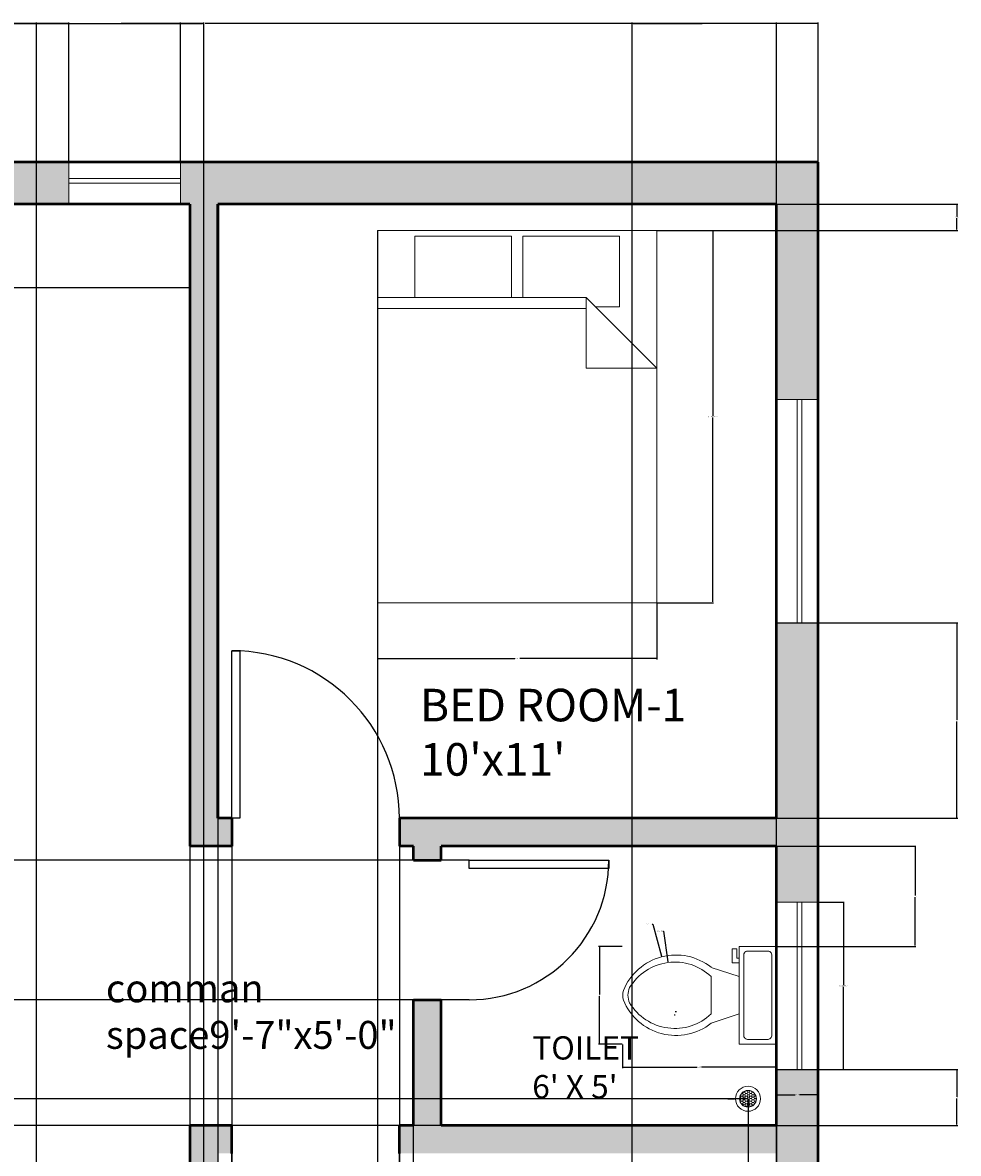
# Model space of a CAD drawing. Units: inches. Extents: x 1489 to 1813, y 1703 to 2293.
# Tile 4 of 4: x 1612 to 1813, y 2050 to 2293. Entities that reach past the tile are written whole.
import ezdxf

# ---------------------------------------------------------------- set-up
doc = ezdxf.new("R2010")
doc.units = ezdxf.units.IN
doc.header["$LTSCALE"] = 0.4
doc.linetypes.add('HIDDEN', pattern=[9.525, 6.35, -3.175])
for name, color, linetype, lineweight in [('A-ANNO-DIMS', 2, 'Continuous', 18), ('A-AREA-IDEN', 7, 'Continuous', 18), ('A-DOOR', 4, 'Continuous', 25), ('A-FIXT-PATT', 8, 'Continuous', 13), ('A-FLOR-CASE', 8, 'Continuous', 25), ('A-FLOR-FIXT', 9, 'Continuous', 18), ('A-FURN', 8, 'Continuous', 18), ('A-GLAZ', 4, 'Continuous', 18), ('A-WALL', 7, 'Continuous', 50)]:
    doc.layers.add(name, color=color, linetype=linetype, lineweight=lineweight)
doc.layers.add('A-WALL-PATT', color=18, linetype='HIDDEN', lineweight=13, true_color=0x000000)
doc.styles.get("Standard").update_dxf_attribs({"font": 'arial.ttf'})
doc.dimstyles.get("Standard").update_dxf_attribs({"dimtxt": 0.18, "dimasz": 0.18, "dimexe": 0.18, "dimexo": 0.0625, "dimgap": 0.09, "dimtad": 0, "dimtih": 1, "dimtoh": 1, "dimdec": 4, "dimzin": 0, "dimdsep": 46, "dimtxsty": 'Standard', "dimcen": 0.09, "dimadec": 0, "dimazin": 0, "dimtfac": 1, "dimtdec": 4, "dimtofl": 0, "dimtmove": 0, "dimatfit": 3, "dimfxl": 1, "dimtolj": 1, "dimtzin": 0, "dimarcsym": 0})

# ---------------------------------------------------------------- blocks, each defined once
blk = doc.blocks.new('*U4')
for p, q in [((0, 0), (0, -6)), ((36, 0), (36, -6))]:
    blk.add_line(p, q)
blk.add_lwpolyline([(0, 0), (0, 36), (1.75, 36), (1.75, 0)], close=True)
blk.add_arc((0, 0), 36, 0, 90)
blk = doc.blocks.new('*U3')
for p, q in [((0, 0), (0, -6)), ((30, 0), (30, -6))]:
    blk.add_line(p, q)
blk.add_lwpolyline([(0, 0), (0, 30), (1.75, 30), (1.75, 0)], close=True)
blk.add_arc((0, 0), 30, 0, 90)
blk = doc.blocks.new('*U5')
for p, q in [((-36, 0), (-36, -6)), ((0, 0), (0, -6))]:
    blk.add_line(p, q)
blk.add_lwpolyline([(0, 0), (0, 36), (-1.75, 36), (-1.75, 0)], close=True)
blk.add_arc((0, 0), 36, 90, 180)
blk = doc.blocks.new('Toilet - top')
for p, q in [((9.5, -6), (9.5, -2)), ((-10, -8.5), (-8, -8.5)), ((-10, -9.5), (-10, -8.5)), ((-7, -9.5), (-10, -9.5)), ((-8, -8.5), (-8, -8)), ((-7, -8), (-7, -9.5)), ((-4, -8), (-6, -14)), ((4, -8), (6, -14)), ((4, -14), (-4, -14))]:
    blk.add_line(p, q)
blk.add_lwpolyline([(10.5, -8), (10.5, 0), (-10.5, 0), (-10.5, -8)], close=True)
for points in [[(-9.5, -2), (-9.5, -6)], [(8.5, -1), (-8.5, -1)], [(-8.5, -7), (8.5, -7)]]:
    blk.add_lwpolyline(points)
for centre, radius, start, end in [((-8.62, -1.88), 0.884, 81.8699, 188.1301), ((8.62, -1.88), 0.884, 351.8699, 98.1301), ((-8.62, -6.12), 0.884, 171.8699, 278.1301), ((8.62, -6.12), 0.884, 261.8699, 8.1301), ((3.52, -21.58), 12.17, 141.4691, 247.9714), ((4.2, -21.82), 11.33, 136.3677, 238.9468), ((-3.52, -21.58), 12.17, 292.0284, 38.5307), ((-4.2, -21.82), 11.33, 301.053, 43.6321), ((0, -27.88), 4, 245.7318, 294.2682), ((0, -29), 4, 254.8605, 285.1395)]:
    blk.add_arc(centre, radius, start, end)
blk = doc.blocks.new('Bed - Queen')
for p, q in [((0, -80.00003), (0, 0)), ((0, 0), (59.99999, 0)), ((59.99999, 0), (59.99999, -80.00003)), ((7.99999, -1.2), (28.79998, -1.2)), ((7.99999, -14.4), (7.99999, -1.2)), ((28.79998, -1.2), (28.79998, -14.4)), ((31.19999, -1.2), (51.99999, -1.2)), ((31.19999, -14.4), (31.19999, -1.2)), ((51.99999, -1.2), (51.99999, -16.4)), ((0, -14.4), (44.8, -14.4)), ((59.99999, -29.6), (44.8, -14.4)), ((44.8, -14.4), (44.8, -29.6)), ((44.8, -16.8), (0, -16.8)), ((51.99999, -16.4), (46.79936, -16.4)), ((44.8, -29.6), (59.99999, -29.6)), ((59.99999, -80.00003), (0, -80.00003))]:
    blk.add_line(p, q)
blk = doc.blocks.new('WIN-48IN')
for p, q in [((9, 48), (0, 48)), ((4.5, 48), (4.5, 0)), ((5.5, 48), (5.5, 0)), ((9, 0), (0, 0))]:
    blk.add_line(p, q)
blk = doc.blocks.new('WIN-36IN')
for p, q in [((0, 36), (9, 36)), ((4.5, 36), (4.5, 0)), ((5.5, 36), (5.5, 0)), ((0, 0), (9, 0))]:
    blk.add_line(p, q)
blk = doc.blocks.new('*D16')
at = {"layer": 'A-ANNO-DIMS', "color": 0, "lineweight": -2, "ltscale": 0.4, "transparency": 16777216}
for p, q in [((1783.05, 2104.17), (1788.56, 2104.17)), ((1788.38, 2103.99), (1788.38, 2086.35)), ((1788.38, 2068.35), (1788.38, 2085.99)), ((1783.05, 2068.17), (1788.56, 2068.17))]:
    blk.add_line(p, q, dxfattribs=at)
at = {"layer": 'A-ANNO-DIMS', "color": 0, "ltscale": 0.4, "transparency": 16777216}
for points in [[(1788.35, 2103.99), (1788.41, 2103.99), (1788.38, 2104.17)], [(1788.35, 2068.35), (1788.41, 2068.35), (1788.38, 2068.17)]]:
    blk.add_solid(points, dxfattribs=at)
at = {"layer": 'Defpoints', "color": 0, "ltscale": 0.4, "transparency": 16777216}
for p in [(1782.98, 2104.17), (1788.38, 2104.17), (1782.98, 2068.17)]:
    blk.add_point(p, dxfattribs=at)
at = {"layer": 'A-ANNO-DIMS', "color": 0, "ltscale": 0.4, "transparency": 16777216, "insert": (1788.38, 2086.17), "char_height": 0.18, "attachment_point": 5}
blk.add_mtext('\\A1;WINDOW 36 TYP.', dxfattribs=at)
blk = doc.blocks.new('*D17')
at = {"layer": 'A-ANNO-DIMS', "color": 0, "lineweight": -2, "ltscale": 0.4, "transparency": 16777216}
for p, q in [((1773.98, 2068.11), (1773.98, 2062.59)), ((1782.98, 2068.11), (1782.98, 2062.59)), ((1774.16, 2062.77), (1778.03, 2062.77)), ((1782.8, 2062.77), (1778.94, 2062.77))]:
    blk.add_line(p, q, dxfattribs=at)
at = {"layer": 'A-ANNO-DIMS', "color": 0, "ltscale": 0.4, "transparency": 16777216}
for points in [[(1774.16, 2062.8), (1774.16, 2062.74), (1773.98, 2062.77)], [(1782.8, 2062.8), (1782.8, 2062.74), (1782.98, 2062.77)]]:
    blk.add_solid(points, dxfattribs=at)
at = {"layer": 'Defpoints', "color": 0, "ltscale": 0.4, "transparency": 16777216}
for p in [(1773.98, 2068.17), (1782.98, 2068.17), (1782.98, 2062.77)]:
    blk.add_point(p, dxfattribs=at)
at = {"layer": 'A-ANNO-DIMS', "color": 0, "ltscale": 0.4, "transparency": 16777216, "insert": (1778.48, 2062.77), "char_height": 0.18, "attachment_point": 5}
blk.add_mtext('\\A1;9 TYP.', dxfattribs=at)
blk = doc.blocks.new('*D18')
at = {"layer": 'A-ANNO-DIMS', "color": 0, "lineweight": -2, "ltscale": 0.4, "transparency": 16777216}
for p, q in [((1748.37, 2248.49), (1760.49, 2248.49)), ((1760.31, 2248.31), (1760.31, 2208.68)), ((1760.31, 2168.67), (1760.31, 2208.3)), ((1748.37, 2168.49), (1760.49, 2168.49))]:
    blk.add_line(p, q, dxfattribs=at)
at = {"layer": 'A-ANNO-DIMS', "color": 0, "ltscale": 0.4, "transparency": 16777216}
for points in [[(1760.28, 2248.31), (1760.34, 2248.31), (1760.31, 2248.49)], [(1760.28, 2168.67), (1760.34, 2168.67), (1760.31, 2168.49)]]:
    blk.add_solid(points, dxfattribs=at)
at = {"layer": 'Defpoints', "color": 0, "ltscale": 0.4, "transparency": 16777216}
for p in [(1748.31, 2248.49), (1760.31, 2248.49), (1748.31, 2168.49)]:
    blk.add_point(p, dxfattribs=at)
at = {"layer": 'A-ANNO-DIMS', "color": 0, "ltscale": 0.4, "transparency": 16777216, "insert": (1760.31, 2208.49), "char_height": 0.18, "attachment_point": 5}
blk.add_mtext('\\A1;QUEEN BED 80 TYP.', dxfattribs=at)
blk = doc.blocks.new('*D19')
at = {"layer": 'A-ANNO-DIMS', "color": 0, "lineweight": -2, "ltscale": 0.4, "transparency": 16777216}
for p, q in [((1688.31, 2168.43), (1688.31, 2156.31)), ((1748.31, 2168.43), (1748.31, 2156.31)), ((1688.49, 2156.49), (1717.78, 2156.49)), ((1748.13, 2156.49), (1718.83, 2156.49))]:
    blk.add_line(p, q, dxfattribs=at)
at = {"layer": 'A-ANNO-DIMS', "color": 0, "ltscale": 0.4, "transparency": 16777216}
for points in [[(1688.49, 2156.52), (1688.49, 2156.46), (1688.31, 2156.49)], [(1748.13, 2156.52), (1748.13, 2156.46), (1748.31, 2156.49)]]:
    blk.add_solid(points, dxfattribs=at)
at = {"layer": 'Defpoints', "color": 0, "ltscale": 0.4, "transparency": 16777216}
for p in [(1688.31, 2168.49), (1748.31, 2168.49), (1748.31, 2156.49)]:
    blk.add_point(p, dxfattribs=at)
at = {"layer": 'A-ANNO-DIMS', "color": 0, "ltscale": 0.4, "transparency": 16777216, "insert": (1718.31, 2156.49), "char_height": 0.18, "attachment_point": 5}
blk.add_mtext('\\A1;60 TYP.', dxfattribs=at)
blk = doc.blocks.new('*D26')
at = {"layer": 'A-ANNO-DIMS', "color": 0, "lineweight": -2, "ltscale": 0.4, "transparency": 16777216}
for p, q in [((1740.94, 2073.59), (1740.94, 2068.51)), ((1773.98, 2073.59), (1773.98, 2068.51)), ((1741.12, 2068.69), (1756.99, 2068.69)), ((1773.8, 2068.69), (1757.93, 2068.69))]:
    blk.add_line(p, q, dxfattribs=at)
at = {"layer": 'A-ANNO-DIMS', "color": 0, "ltscale": 0.4, "transparency": 16777216}
for points in [[(1741.12, 2068.72), (1741.12, 2068.66), (1740.94, 2068.69)], [(1773.8, 2068.72), (1773.8, 2068.66), (1773.98, 2068.69)]]:
    blk.add_solid(points, dxfattribs=at)
at = {"layer": 'Defpoints', "color": 0, "ltscale": 0.4, "transparency": 16777216}
for p in [(1740.94, 2073.65), (1773.98, 2073.65), (1773.98, 2068.69)]:
    blk.add_point(p, dxfattribs=at)
at = {"layer": 'A-ANNO-DIMS', "color": 0, "ltscale": 0.4, "transparency": 16777216, "insert": (1757.46, 2068.69), "char_height": 0.18, "attachment_point": 5}
blk.add_mtext('\\A1;WC 33', dxfattribs=at)
blk = doc.blocks.new('*D27')
at = {"layer": 'A-ANNO-DIMS', "color": 0, "lineweight": -2, "ltscale": 0.4, "transparency": 16777216}
for p, q in [((1740.88, 2094.65), (1735.8, 2094.65)), ((1735.98, 2094.47), (1735.98, 2084.33)), ((1735.98, 2073.83), (1735.98, 2083.97)), ((1740.88, 2073.65), (1735.8, 2073.65))]:
    blk.add_line(p, q, dxfattribs=at)
at = {"layer": 'A-ANNO-DIMS', "color": 0, "ltscale": 0.4, "transparency": 16777216}
for points in [[(1735.95, 2094.47), (1736.01, 2094.47), (1735.98, 2094.65)], [(1735.95, 2073.83), (1736.01, 2073.83), (1735.98, 2073.65)]]:
    blk.add_solid(points, dxfattribs=at)
at = {"layer": 'Defpoints', "color": 0, "ltscale": 0.4, "transparency": 16777216}
for p in [(1740.94, 2094.65), (1735.98, 2073.65), (1740.94, 2073.65)]:
    blk.add_point(p, dxfattribs=at)
at = {"layer": 'A-ANNO-DIMS', "color": 0, "ltscale": 0.4, "transparency": 16777216, "insert": (1735.98, 2084.15), "char_height": 0.18, "attachment_point": 5}
blk.add_mtext('\\A1;21', dxfattribs=at)
blk = doc.blocks.new('*D28')
at = {"layer": 'A-ANNO-DIMS', "color": 0, "lineweight": -2, "ltscale": 0.4, "transparency": 16777216}
for p, q in [((1518.98, 2263.23), (1518.98, 2293.15)), ((1519.16, 2292.97), (1650.69, 2292.97)), ((1782.8, 2292.97), (1651.27, 2292.97)), ((1782.98, 2263.23), (1782.98, 2293.15))]:
    blk.add_line(p, q, dxfattribs=at)
at = {"layer": 'A-ANNO-DIMS', "color": 0, "ltscale": 0.4, "transparency": 16777216}
for points in [[(1519.16, 2293), (1519.16, 2292.94), (1518.98, 2292.97)], [(1782.8, 2293), (1782.8, 2292.94), (1782.98, 2292.97)]]:
    blk.add_solid(points, dxfattribs=at)
at = {"layer": 'Defpoints', "color": 0, "ltscale": 0.4, "transparency": 16777216}
for p in [(1782.98, 2292.97), (1518.98, 2263.17), (1782.98, 2263.17)]:
    blk.add_point(p, dxfattribs=at)
at = {"layer": 'A-ANNO-DIMS', "color": 0, "ltscale": 0.4, "transparency": 16777216, "insert": (1650.98, 2292.97), "char_height": 0.18, "attachment_point": 5}
blk.add_mtext('\\A1;264', dxfattribs=at)
blk = doc.blocks.new('*D33')
at = {"layer": 'A-ANNO-DIMS', "color": 0, "lineweight": -2, "ltscale": 0.4, "transparency": 16777216}
for p, q in [((1614.98, 1783.23), (1614.98, 2293.15)), ((1615.16, 2292.97), (1632.77, 2292.97)), ((1650.8, 2292.97), (1633.2, 2292.97)), ((1650.98, 1783.23), (1650.98, 2293.15))]:
    blk.add_line(p, q, dxfattribs=at)
at = {"layer": 'A-ANNO-DIMS', "color": 0, "ltscale": 0.4, "transparency": 16777216}
for points in [[(1615.16, 2293), (1615.16, 2292.94), (1614.98, 2292.97)], [(1650.8, 2293), (1650.8, 2292.94), (1650.98, 2292.97)]]:
    blk.add_solid(points, dxfattribs=at)
at = {"layer": 'Defpoints', "color": 0, "ltscale": 0.4, "transparency": 16777216}
for p in [(1650.98, 2292.97), (1614.98, 1783.17), (1650.98, 1783.17)]:
    blk.add_point(p, dxfattribs=at)
at = {"layer": 'A-ANNO-DIMS', "color": 0, "ltscale": 0.4, "transparency": 16777216, "insert": (1632.98, 2292.97), "char_height": 0.18, "attachment_point": 5}
blk.add_mtext('\\A1;36', dxfattribs=at)
blk = doc.blocks.new('*D38')
at = {"layer": 'A-ANNO-DIMS', "color": 0, "lineweight": -2, "ltscale": 0.4, "transparency": 16777216}
for p, q in [((1774.05, 2164.17), (1812.96, 2164.17)), ((1812.78, 2163.99), (1812.78, 2143.35)), ((1812.78, 2122.35), (1812.78, 2142.99)), ((1774.05, 2122.17), (1812.96, 2122.17))]:
    blk.add_line(p, q, dxfattribs=at)
at = {"layer": 'A-ANNO-DIMS', "color": 0, "ltscale": 0.4, "transparency": 16777216}
for points in [[(1812.75, 2163.99), (1812.81, 2163.99), (1812.78, 2164.17)], [(1812.75, 2122.35), (1812.81, 2122.35), (1812.78, 2122.17)]]:
    blk.add_solid(points, dxfattribs=at)
at = {"layer": 'Defpoints', "color": 0, "ltscale": 0.4, "transparency": 16777216}
for p in [(1773.98, 2164.17), (1812.78, 2164.17), (1773.98, 2122.17)]:
    blk.add_point(p, dxfattribs=at)
at = {"layer": 'A-ANNO-DIMS', "color": 0, "ltscale": 0.4, "transparency": 16777216, "insert": (1812.78, 2143.17), "char_height": 0.18, "attachment_point": 5}
blk.add_mtext('\\A1;42', dxfattribs=at)
blk = doc.blocks.new('*D39')
at = {"layer": 'A-ANNO-DIMS', "color": 0, "lineweight": -2, "ltscale": 0.4, "transparency": 16777216}
for p, q in [((1518.98, 2263.23), (1518.98, 2293.15)), ((1519.16, 2292.97), (1570.2, 2292.97)), ((1621.8, 2292.97), (1570.76, 2292.97)), ((1621.98, 2263.23), (1621.98, 2293.15))]:
    blk.add_line(p, q, dxfattribs=at)
at = {"layer": 'A-ANNO-DIMS', "color": 0, "ltscale": 0.4, "transparency": 16777216}
for points in [[(1519.16, 2293), (1519.16, 2292.94), (1518.98, 2292.97)], [(1621.8, 2293), (1621.8, 2292.94), (1621.98, 2292.97)]]:
    blk.add_solid(points, dxfattribs=at)
at = {"layer": 'Defpoints', "color": 0, "ltscale": 0.4, "transparency": 16777216}
for p in [(1621.98, 2292.97), (1518.98, 2263.17), (1621.98, 2263.17)]:
    blk.add_point(p, dxfattribs=at)
at = {"layer": 'A-ANNO-DIMS', "color": 0, "ltscale": 0.4, "transparency": 16777216, "insert": (1570.48, 2292.97), "char_height": 0.18, "attachment_point": 5}
blk.add_mtext('\\A1;103', dxfattribs=at)
blk = doc.blocks.new('*D40')
at = {"layer": 'A-ANNO-DIMS', "color": 0, "lineweight": -2, "ltscale": 0.4, "transparency": 16777216}
for p, q in [((1621.98, 2263.23), (1621.98, 2293.15)), ((1622.16, 2292.97), (1633.76, 2292.97)), ((1645.8, 2292.97), (1634.2, 2292.97)), ((1645.98, 2263.23), (1645.98, 2293.15))]:
    blk.add_line(p, q, dxfattribs=at)
at = {"layer": 'A-ANNO-DIMS', "color": 0, "ltscale": 0.4, "transparency": 16777216}
for points in [[(1622.16, 2293), (1622.16, 2292.94), (1621.98, 2292.97)], [(1645.8, 2293), (1645.8, 2292.94), (1645.98, 2292.97)]]:
    blk.add_solid(points, dxfattribs=at)
at = {"layer": 'Defpoints', "color": 0, "ltscale": 0.4, "transparency": 16777216}
for p in [(1645.98, 2292.97), (1621.98, 2263.17), (1645.98, 2263.17)]:
    blk.add_point(p, dxfattribs=at)
at = {"layer": 'A-ANNO-DIMS', "color": 0, "ltscale": 0.4, "transparency": 16777216, "insert": (1633.98, 2292.97), "char_height": 0.18, "attachment_point": 5}
blk.add_mtext('\\A1;24', dxfattribs=at)
blk = doc.blocks.new('*D41')
at = {"layer": 'A-ANNO-DIMS', "color": 0, "lineweight": -2, "ltscale": 0.4, "transparency": 16777216}
for p, q in [((1647.98, 2254.11), (1647.98, 1705.95)), ((1653.98, 2254.11), (1653.98, 1705.95)), ((1648.16, 1706.13), (1650.83, 1706.13)), ((1653.8, 1706.13), (1651.13, 1706.13))]:
    blk.add_line(p, q, dxfattribs=at)
at = {"layer": 'A-ANNO-DIMS', "color": 0, "ltscale": 0.4, "transparency": 16777216}
for points in [[(1648.16, 1706.16), (1648.16, 1706.1), (1647.98, 1706.13)], [(1653.8, 1706.16), (1653.8, 1706.1), (1653.98, 1706.13)]]:
    blk.add_solid(points, dxfattribs=at)
at = {"layer": 'Defpoints', "color": 0, "ltscale": 0.4, "transparency": 16777216}
for p in [(1647.98, 2254.17), (1653.98, 2254.17), (1653.98, 1706.13)]:
    blk.add_point(p, dxfattribs=at)
at = {"layer": 'A-ANNO-DIMS', "color": 0, "ltscale": 0.4, "transparency": 16777216, "insert": (1650.98, 1706.13), "char_height": 0.18, "attachment_point": 5}
blk.add_mtext('\\A1;6', dxfattribs=at)
blk = doc.blocks.new('*D46')
at = {"layer": 'A-ANNO-DIMS', "color": 0, "lineweight": -2, "ltscale": 0.4, "transparency": 16777216}
for p, q in [((1774.05, 2068.17), (1812.96, 2068.17)), ((1812.78, 2067.99), (1812.78, 2062.35)), ((1812.78, 2056.35), (1812.78, 2061.99)), ((1774.05, 2056.17), (1812.96, 2056.17))]:
    blk.add_line(p, q, dxfattribs=at)
at = {"layer": 'A-ANNO-DIMS', "color": 0, "ltscale": 0.4, "transparency": 16777216}
for points in [[(1812.75, 2067.99), (1812.81, 2067.99), (1812.78, 2068.17)], [(1812.75, 2056.35), (1812.81, 2056.35), (1812.78, 2056.17)]]:
    blk.add_solid(points, dxfattribs=at)
at = {"layer": 'Defpoints', "color": 0, "ltscale": 0.4, "transparency": 16777216}
for p in [(1773.98, 2068.17), (1812.78, 2068.17), (1773.98, 2056.17)]:
    blk.add_point(p, dxfattribs=at)
at = {"layer": 'A-ANNO-DIMS', "color": 0, "ltscale": 0.4, "transparency": 16777216, "insert": (1812.78, 2062.17), "char_height": 0.18, "attachment_point": 5}
blk.add_mtext('\\A1;12', dxfattribs=at)
blk = doc.blocks.new('*D47')
at = {"layer": 'A-ANNO-DIMS', "color": 0, "lineweight": -2, "ltscale": 0.4, "transparency": 16777216}
for p, q in [((1701.92, 2113.17), (1489, 2113.17)), ((1489.18, 2112.99), (1489.18, 2098.35)), ((1489.18, 2083.35), (1489.18, 2097.99)), ((1701.92, 2083.17), (1489, 2083.17))]:
    blk.add_line(p, q, dxfattribs=at)
at = {"layer": 'A-ANNO-DIMS', "color": 0, "ltscale": 0.4, "transparency": 16777216}
for points in [[(1489.15, 2112.99), (1489.21, 2112.99), (1489.18, 2113.17)], [(1489.15, 2083.35), (1489.21, 2083.35), (1489.18, 2083.17)]]:
    blk.add_solid(points, dxfattribs=at)
at = {"layer": 'Defpoints', "color": 0, "ltscale": 0.4, "transparency": 16777216}
for p in [(1701.98, 2113.17), (1489.18, 2083.17), (1701.98, 2083.17)]:
    blk.add_point(p, dxfattribs=at)
at = {"layer": 'A-ANNO-DIMS', "color": 0, "ltscale": 0.4, "transparency": 16777216, "insert": (1489.18, 2098.17), "char_height": 0.18, "attachment_point": 5}
blk.add_mtext('\\A1;30', dxfattribs=at)
blk = doc.blocks.new('*D49')
at = {"layer": 'A-ANNO-DIMS', "color": 0, "lineweight": -2, "ltscale": 0.4, "transparency": 16777216}
for p, q in [((1743, 1846.23), (1743, 2293.15)), ((1743.18, 2292.97), (1758.03, 2292.97)), ((1773.8, 2292.97), (1758.96, 2292.97)), ((1773.98, 1846.23), (1773.98, 2293.15))]:
    blk.add_line(p, q, dxfattribs=at)
at = {"layer": 'A-ANNO-DIMS', "color": 0, "ltscale": 0.4, "transparency": 16777216}
for points in [[(1743.18, 2293), (1743.18, 2292.94), (1743, 2292.97)], [(1773.8, 2293), (1773.8, 2292.94), (1773.98, 2292.97)]]:
    blk.add_solid(points, dxfattribs=at)
at = {"layer": 'Defpoints', "color": 0, "ltscale": 0.4, "transparency": 16777216}
for p in [(1773.98, 2292.97), (1743, 1846.17), (1773.98, 1846.17)]:
    blk.add_point(p, dxfattribs=at)
at = {"layer": 'A-ANNO-DIMS', "color": 0, "ltscale": 0.4, "transparency": 16777216, "insert": (1758.49, 2292.97), "char_height": 0.18, "attachment_point": 5}
blk.add_mtext('\\A1;30.983', dxfattribs=at)
blk = doc.blocks.new('*D53')
at = {"layer": 'A-ANNO-DIMS', "color": 0, "lineweight": -2, "ltscale": 0.4, "transparency": 16777216}
for p, q in [((1656.98, 2122.11), (1656.98, 1705.95)), ((1692.98, 2122.11), (1692.98, 1705.95)), ((1657.16, 1706.13), (1674.77, 1706.13)), ((1692.8, 1706.13), (1675.2, 1706.13))]:
    blk.add_line(p, q, dxfattribs=at)
at = {"layer": 'A-ANNO-DIMS', "color": 0, "ltscale": 0.4, "transparency": 16777216}
for points in [[(1657.16, 1706.16), (1657.16, 1706.1), (1656.98, 1706.13)], [(1692.8, 1706.16), (1692.8, 1706.1), (1692.98, 1706.13)]]:
    blk.add_solid(points, dxfattribs=at)
at = {"layer": 'Defpoints', "color": 0, "ltscale": 0.4, "transparency": 16777216}
for p in [(1656.98, 2122.17), (1692.98, 2122.17), (1692.98, 1706.13)]:
    blk.add_point(p, dxfattribs=at)
at = {"layer": 'A-ANNO-DIMS', "color": 0, "ltscale": 0.4, "transparency": 16777216, "insert": (1674.98, 1706.13), "char_height": 0.18, "attachment_point": 5}
blk.add_mtext('\\A1;36', dxfattribs=at)
blk = doc.blocks.new('*D58')
at = {"layer": 'A-ANNO-DIMS', "color": 0, "lineweight": -2, "ltscale": 0.4, "transparency": 16777216}
for p, q in [((1774.05, 2116.17), (1803.96, 2116.17)), ((1803.78, 2115.99), (1803.78, 2105.59)), ((1803.78, 2094.83), (1803.78, 2105.23)), ((1774.05, 2094.65), (1803.96, 2094.65))]:
    blk.add_line(p, q, dxfattribs=at)
at = {"layer": 'A-ANNO-DIMS', "color": 0, "ltscale": 0.4, "transparency": 16777216}
for points in [[(1803.75, 2115.99), (1803.81, 2115.99), (1803.78, 2116.17)], [(1803.75, 2094.83), (1803.81, 2094.83), (1803.78, 2094.65)]]:
    blk.add_solid(points, dxfattribs=at)
at = {"layer": 'Defpoints', "color": 0, "ltscale": 0.4, "transparency": 16777216}
for p in [(1773.98, 2116.17), (1773.98, 2094.65), (1803.78, 2094.65)]:
    blk.add_point(p, dxfattribs=at)
at = {"layer": 'A-ANNO-DIMS', "color": 0, "ltscale": 0.4, "transparency": 16777216, "insert": (1803.78, 2105.41), "char_height": 0.18, "attachment_point": 5}
blk.add_mtext('\\A1;21.52', dxfattribs=at)
blk = doc.blocks.new('*D59')
at = {"layer": 'A-ANNO-DIMS', "color": 0, "lineweight": -2, "ltscale": 0.4, "transparency": 16777216}
for p, q in [((1653.98, 2254.11), (1653.98, 1705.95)), ((1688.31, 2248.43), (1688.31, 1705.95)), ((1654.16, 1706.13), (1670.75, 1706.13)), ((1688.13, 1706.13), (1671.54, 1706.13))]:
    blk.add_line(p, q, dxfattribs=at)
at = {"layer": 'A-ANNO-DIMS', "color": 0, "ltscale": 0.4, "transparency": 16777216}
for points in [[(1654.16, 1706.16), (1654.16, 1706.1), (1653.98, 1706.13)], [(1688.13, 1706.16), (1688.13, 1706.1), (1688.31, 1706.13)]]:
    blk.add_solid(points, dxfattribs=at)
at = {"layer": 'Defpoints', "color": 0, "ltscale": 0.4, "transparency": 16777216}
for p in [(1653.98, 2254.17), (1688.31, 2248.49), (1688.31, 1706.13)]:
    blk.add_point(p, dxfattribs=at)
at = {"layer": 'A-ANNO-DIMS', "color": 0, "ltscale": 0.4, "transparency": 16777216, "insert": (1671.14, 1706.13), "char_height": 0.18, "attachment_point": 5}
blk.add_mtext('\\A1;34.32', dxfattribs=at)
blk = doc.blocks.new('*D60')
at = {"layer": 'A-ANNO-DIMS', "color": 0, "lineweight": -2, "ltscale": 0.4, "transparency": 16777216}
for p, q in [((1774.05, 2254.17), (1812.96, 2254.17)), ((1812.78, 2253.99), (1812.78, 2251.51)), ((1812.78, 2248.67), (1812.78, 2251.15)), ((1748.37, 2248.49), (1812.96, 2248.49))]:
    blk.add_line(p, q, dxfattribs=at)
at = {"layer": 'A-ANNO-DIMS', "color": 0, "ltscale": 0.4, "transparency": 16777216}
for points in [[(1812.75, 2253.99), (1812.81, 2253.99), (1812.78, 2254.17)], [(1812.75, 2248.67), (1812.81, 2248.67), (1812.78, 2248.49)]]:
    blk.add_solid(points, dxfattribs=at)
at = {"layer": 'Defpoints', "color": 0, "ltscale": 0.4, "transparency": 16777216}
for p in [(1773.98, 2254.17), (1812.78, 2254.17), (1748.31, 2248.49)]:
    blk.add_point(p, dxfattribs=at)
at = {"layer": 'A-ANNO-DIMS', "color": 0, "ltscale": 0.4, "transparency": 16777216, "insert": (1812.78, 2251.33), "char_height": 0.18, "attachment_point": 5}
blk.add_mtext('\\A1;5.678', dxfattribs=at)
blk = doc.blocks.new('*D63')
at = {"layer": 'A-ANNO-DIMS', "color": 0, "lineweight": -2, "ltscale": 0.4, "transparency": 16777216}
for p, q in [((1581.98, 2062.11), (1581.98, 1705.95)), ((1695.98, 2056.11), (1695.98, 1705.95)), ((1582.16, 1706.13), (1638.7, 1706.13)), ((1695.8, 1706.13), (1639.26, 1706.13))]:
    blk.add_line(p, q, dxfattribs=at)
at = {"layer": 'A-ANNO-DIMS', "color": 0, "ltscale": 0.4, "transparency": 16777216}
for points in [[(1582.16, 1706.16), (1582.16, 1706.1), (1581.98, 1706.13)], [(1695.8, 1706.16), (1695.8, 1706.1), (1695.98, 1706.13)]]:
    blk.add_solid(points, dxfattribs=at)
at = {"layer": 'Defpoints', "color": 0, "ltscale": 0.4, "transparency": 16777216}
for p in [(1581.98, 2062.17), (1695.98, 2056.17), (1695.98, 1706.13)]:
    blk.add_point(p, dxfattribs=at)
at = {"layer": 'A-ANNO-DIMS', "color": 0, "ltscale": 0.4, "transparency": 16777216, "insert": (1638.98, 1706.13), "char_height": 0.18, "attachment_point": 5}
blk.add_mtext('\\A1;114', dxfattribs=at)
blk = doc.blocks.new('*D64')
at = {"layer": 'A-ANNO-DIMS', "color": 0, "lineweight": -2, "ltscale": 0.4, "transparency": 16777216}
for p, q in [((1767.89, 2061.85), (1767.89, 1705.95)), ((1773.98, 2056.11), (1773.98, 1705.95)), ((1768.07, 1706.13), (1770.56, 1706.13)), ((1773.8, 1706.13), (1771.31, 1706.13))]:
    blk.add_line(p, q, dxfattribs=at)
at = {"layer": 'A-ANNO-DIMS', "color": 0, "ltscale": 0.4, "transparency": 16777216}
for points in [[(1768.07, 1706.16), (1768.07, 1706.1), (1767.89, 1706.13)], [(1773.8, 1706.16), (1773.8, 1706.1), (1773.98, 1706.13)]]:
    blk.add_solid(points, dxfattribs=at)
at = {"layer": 'Defpoints', "color": 0, "ltscale": 0.4, "transparency": 16777216}
for p in [(1767.89, 2061.91), (1773.98, 2056.17), (1773.98, 1706.13)]:
    blk.add_point(p, dxfattribs=at)
at = {"layer": 'A-ANNO-DIMS', "color": 0, "ltscale": 0.4, "transparency": 16777216, "insert": (1770.94, 1706.13), "char_height": 0.18, "attachment_point": 5}
blk.add_mtext('\\A1;6.091', dxfattribs=at)
blk = doc.blocks.new('*D65')
at = {"layer": 'A-ANNO-DIMS', "color": 0, "lineweight": -2, "ltscale": 0.4, "transparency": 16777216}
for p, q in [((1767.83, 2061.91), (1489, 2061.91)), ((1489.18, 2061.73), (1489.18, 2059.22)), ((1489.18, 2056.35), (1489.18, 2058.86)), ((1773.92, 2056.17), (1489, 2056.17))]:
    blk.add_line(p, q, dxfattribs=at)
at = {"layer": 'A-ANNO-DIMS', "color": 0, "ltscale": 0.4, "transparency": 16777216}
for points in [[(1489.15, 2061.73), (1489.21, 2061.73), (1489.18, 2061.91)], [(1489.15, 2056.35), (1489.21, 2056.35), (1489.18, 2056.17)]]:
    blk.add_solid(points, dxfattribs=at)
at = {"layer": 'Defpoints', "color": 0, "ltscale": 0.4, "transparency": 16777216}
for p in [(1767.89, 2061.91), (1489.18, 2056.17), (1773.98, 2056.17)]:
    blk.add_point(p, dxfattribs=at)
at = {"layer": 'A-ANNO-DIMS', "color": 0, "ltscale": 0.4, "transparency": 16777216, "insert": (1489.18, 2059.04), "char_height": 0.18, "attachment_point": 5}
blk.add_mtext('\\A1;5.74', dxfattribs=at)
blk = doc.blocks.new('*D66')
at = {"layer": 'A-ANNO-DIMS', "color": 0, "lineweight": -2, "ltscale": 0.4, "transparency": 16777216}
for p, q in [((1747.28, 2099.46), (1747.46, 2099.46)), ((1747.46, 2099.46), (1749.27, 2092.57)), ((1752.31, 2080.63), (1752.49, 2080.63)), ((1752.4, 2080.54), (1752.4, 2080.72))]:
    blk.add_line(p, q, dxfattribs=at)
at = {"layer": 'A-ANNO-DIMS', "color": 0, "ltscale": 0.4, "transparency": 16777216}
blk.add_solid([(1749.29, 2092.58), (1749.24, 2092.57), (1749.31, 2092.4)], dxfattribs=at)
at = {"layer": 'Defpoints', "color": 0, "ltscale": 0.4, "transparency": 16777216}
for p in [(1749.31, 2092.4), (1752.4, 2080.63)]:
    blk.add_point(p, dxfattribs=at)
at = {"layer": 'A-ANNO-DIMS', "color": 0, "ltscale": 0.4, "transparency": 16777216, "insert": (1746.6, 2099.46), "char_height": 0.18, "attachment_point": 5}
blk.add_mtext('\\A1;2X R12.17', dxfattribs=at)
blk = doc.blocks.new('*D67')
at = {"layer": 'A-ANNO-DIMS', "color": 0, "lineweight": -2, "ltscale": 0.4, "transparency": 16777216}
for p, q in [((1749.57, 2097.91), (1749.75, 2097.91)), ((1749.75, 2097.91), (1750.63, 2091.36)), ((1752.08, 2079.95), (1752.26, 2079.95)), ((1752.17, 2079.86), (1752.17, 2080.04))]:
    blk.add_line(p, q, dxfattribs=at)
at = {"layer": 'A-ANNO-DIMS', "color": 0, "ltscale": 0.4, "transparency": 16777216}
blk.add_solid([(1750.66, 2091.36), (1750.6, 2091.35), (1750.66, 2091.18)], dxfattribs=at)
at = {"layer": 'Defpoints', "color": 0, "ltscale": 0.4, "transparency": 16777216}
for p in [(1750.66, 2091.18), (1752.17, 2079.95)]:
    blk.add_point(p, dxfattribs=at)
at = {"layer": 'A-ANNO-DIMS', "color": 0, "ltscale": 0.4, "transparency": 16777216, "insert": (1748.9, 2097.91), "char_height": 0.18, "attachment_point": 5}
blk.add_mtext('\\A1;2X R11.33', dxfattribs=at)
blk = doc.blocks.new('*D68')
at = {"layer": 'A-ANNO-DIMS', "color": 0, "lineweight": -2, "ltscale": 0.4, "transparency": 16777216}
for p, q in [((1763.59, 2061.91), (1765.02, 2061.91)), ((1767.8, 2061.91), (1767.98, 2061.91)), ((1767.89, 2061.82), (1767.89, 2062))]:
    blk.add_line(p, q, dxfattribs=at)
at = {"layer": 'A-ANNO-DIMS', "color": 0, "ltscale": 0.4, "transparency": 16777216}
blk.add_solid([(1765.02, 2061.94), (1765.02, 2061.88), (1765.2, 2061.91)], dxfattribs=at)
at = {"layer": 'Defpoints', "color": 0, "ltscale": 0.4, "transparency": 16777216}
for p in [(1765.2, 2061.91), (1770.58, 2061.91)]:
    blk.add_point(p, dxfattribs=at)
at = {"layer": 'A-ANNO-DIMS', "color": 0, "ltscale": 0.4, "transparency": 16777216, "insert": (1763.1, 2061.91), "char_height": 0.18, "attachment_point": 5}
blk.add_mtext('\\A1;∅5.375', dxfattribs=at)

msp = doc.modelspace()

# ---------------------------------------------------------------- hatches: boundary and pattern name
at = {"layer": 'A-FIXT-PATT'}
h = msp.add_hatch(dxfattribs=at)
h.set_pattern_fill('HONEY', color=256, scale=0.1)
h.paths.add_polyline_path([(1766.0849, 2061.9104, 1), (1769.7, 2061.9104, 1)])
at = {"layer": 'A-WALL-PATT', "ltscale": 0.4}
h = msp.add_hatch(dxfattribs=at)
h.set_pattern_fill('HONEY', color=256, scale=0.1)
h.paths.add_polyline_path([(1621.9839, 2263.1709), (1518.9839, 2263.1709), (1518.9839, 2218.1709), (1527.9839, 2218.1709), (1527.9839, 2254.1709), (1621.9839, 2254.1709)])
h = msp.add_hatch(dxfattribs=at)
h.set_pattern_fill('HONEY', color=256, scale=0.1)
h.paths.add_polyline_path([(1782.9839, 2263.1709), (1645.9839, 2263.1709), (1645.9839, 2254.1709), (1647.9839, 2254.1709), (1647.9839, 2116.1709), (1653.9839, 2116.1709), (1656.9839, 2116.1709), (1656.9839, 2122.1709), (1653.9839, 2122.1709), (1653.9839, 2254.1709), (1773.9839, 2254.1709), (1773.9839, 2212.1709), (1782.9839, 2212.1709)])
h.paths.add_polyline_path([(1782.9839, 2164.1709), (1773.9839, 2164.1709), (1773.9839, 2122.1709), (1695.9839, 2122.1709), (1692.9839, 2122.1709), (1692.9839, 2116.1709), (1695.9839, 2116.1709), (1695.9839, 2113.1709), (1701.9839, 2113.1709), (1701.9839, 2116.1709), (1773.9839, 2116.1709), (1773.9839, 2104.1709), (1782.9839, 2104.1709)])
h.paths.add_polyline_path([(1782.9839, 2068.1709), (1773.9839, 2068.1709), (1773.9839, 2056.1709), (1701.9839, 2056.1709), (1701.9839, 2083.1709), (1695.9839, 2083.1709), (1695.9839, 2056.1709), (1692.9839, 2056.1709), (1692.9839, 2050.1709), (1695.9839, 2050.1709), (1773.9839, 2050.1709), (1773.9839, 2014.1709), (1782.9839, 2014.1709)])
h = msp.add_hatch(dxfattribs=at)
h.set_pattern_fill('HONEY', color=256, scale=0.1)
h.paths.add_polyline_path([(1653.9839, 2050.1709), (1656.9839, 2050.1709), (1656.9839, 2056.1709), (1653.9839, 2056.1709), (1647.9839, 2056.1709), (1647.9839, 1930.1709), (1644.9839, 1930.1709), (1644.9839, 1924.1709), (1773.9839, 1924.1709), (1773.9839, 1903.1709), (1782.9839, 1903.1709), (1782.9839, 1966.1709), (1773.9839, 1966.1709), (1773.9839, 1930.1709), (1653.9839, 1930.1709)])

# ---------------------------------------------------------------- linework, layer by layer
at = {"layer": 'A-FLOR-CASE'}
msp.add_line((1647.9839, 2236.1709), (1545.9839, 2236.1709), dxfattribs=at)
at = {"layer": 'A-FLOR-FIXT'}
for radius in [2.6876, 1.8076]:
    msp.add_circle((1767.8924, 2061.9104), radius, dxfattribs=at)
at = {"layer": 'A-GLAZ'}
for p, q in [((1621.9839, 2254.1709), (1621.9839, 2263.1709)), ((1645.9839, 2254.1709), (1645.9839, 2263.1709)), ((1621.9839, 2259.6709), (1645.9839, 2259.6709)), ((1621.9839, 2258.6709), (1645.9839, 2258.6709))]:
    msp.add_line(p, q, dxfattribs=at)
at = {"layer": 'A-WALL'}
for p, q in [((1782.9839, 2263.1709), (1518.9839, 2263.1709)), ((1782.9839, 1783.1709), (1782.9839, 2263.1709)), ((1647.9839, 2254.1709), (1527.9839, 2254.1709)), ((1647.9839, 2254.1709), (1647.9839, 2116.1709)), ((1773.9839, 2254.1709), (1653.9839, 2254.1709)), ((1653.9839, 2254.1709), (1653.9839, 2122.1709)), ((1653.9839, 2122.1709), (1653.9839, 2254.1709)), ((1773.9839, 2122.1709), (1773.9839, 2254.1709)), ((1656.9839, 2122.1709), (1653.9839, 2122.1709)), ((1656.9839, 2122.1709), (1656.9839, 2116.1709)), ((1695.9839, 2122.1709), (1692.9839, 2122.1709)), ((1692.9839, 2122.1709), (1692.9839, 2116.1709)), ((1773.9839, 2122.1709), (1695.9839, 2122.1709)), ((1653.9839, 2116.1709), (1647.9839, 2116.1709)), ((1656.9839, 2116.1709), (1653.9839, 2116.1709)), ((1695.9839, 2116.1709), (1692.9839, 2116.1709)), ((1695.9839, 2113.1709), (1695.9839, 2116.1709)), ((1773.9839, 2116.1709), (1701.9839, 2116.1709)), ((1701.9839, 2113.1709), (1701.9839, 2116.1709)), ((1773.9839, 2056.1709), (1773.9839, 2116.1709)), ((1695.9839, 2113.1709), (1701.9839, 2113.1709)), ((1695.9839, 2056.1709), (1695.9839, 2083.1709)), ((1695.9839, 2083.1709), (1701.9839, 2083.1709)), ((1701.9839, 2056.1709), (1701.9839, 2083.1709)), ((1653.9839, 2056.1709), (1647.9839, 2056.1709)), ((1647.9839, 2056.1709), (1647.9839, 1930.1709)), ((1656.9839, 2056.1709), (1653.9839, 2056.1709)), ((1656.9839, 2050.1709), (1656.9839, 2056.1709)), ((1695.9839, 2056.1709), (1692.9839, 2056.1709)), ((1692.9839, 2050.1709), (1692.9839, 2056.1709)), ((1773.9839, 2056.1709), (1701.9839, 2056.1709))]:
    msp.add_line(p, q, dxfattribs=at)

# ---------------------------------------------------------------- block references
at = {"layer": 'A-DOOR'}
msp.add_blockref('*U4', (1656.9839, 2122.1709), dxfattribs=at)
for name, p, rotation in [('*U3', (1707.9839, 2113.1709), 270), ('*U5', (1656.9839, 2044.1709), 180)]:
    msp.add_blockref(name, p, dxfattribs=dict(at, rotation=rotation))
at = {"layer": 'A-FLOR-FIXT', "rotation": 270}
msp.add_blockref('Toilet - top', (1773.9839, 2084.1496), dxfattribs=at)
at = {"layer": 'A-FURN'}
msp.add_blockref('Bed - Queen', (1688.3051, 2248.4927), dxfattribs=at)
at = {"layer": 'A-GLAZ'}
for name, p in [('WIN-48IN', (1773.984, 2164.171)), ('WIN-36IN', (1773.984, 2068.171))]:
    msp.add_blockref(name, p, dxfattribs=at)

# ---------------------------------------------------------------- texts
at = {"layer": 'A-AREA-IDEN', "attachment_point": 1}
for s, width, insert, char_height in [("BED ROOM-1\\P10'x11'", 87.866044, (1697.4044, 2150.0034), 7), ('comman space9\'-7"x5\'-0"', 61.598528, (1629.9278, 2088.6352), 6), ("TOILET\\P6' X 5'", 19.077425, (1721.5298, 2075.3377), 5)]:
    msp.add_mtext_dynamic_manual_height_columns(s, width=width, gutter_width=12.5, heights=[0], dxfattribs=dict(at, insert=insert, char_height=char_height))

# ---------------------------------------------------------------- dimensions: what is measured, and where the dimension line sits
at = {"layer": 'A-ANNO-DIMS', "ltscale": 0.4}
for base, p1, p2, override, picture, middle in [((1782.9839, 2292.9709), (1518.9839, 2263.1709), (1782.9839, 2263.1709), {"dimdec": 0, "dimlfac": 1, "dimrnd": 0, "dimzin": 0, "dimdsep": 46, "dimlunit": 2}, '*D28', (1650.9839, 2292.9709)), ((1621.9839, 2292.9709), (1518.9839, 2263.1709), (1621.9839, 2263.1709), {"dimdec": 0, "dimlfac": 1, "dimrnd": 0, "dimzin": 0, "dimdsep": 46, "dimlunit": 2}, '*D39', (1570.4839, 2292.9709)), ((1650.9839, 2292.9709), (1614.9839, 1783.1709), (1650.9839, 1783.1709), {"dimdec": 0, "dimlfac": 1, "dimrnd": 0, "dimzin": 0, "dimdsep": 46, "dimlunit": 2}, '*D33', (1632.9839, 2292.9709)), ((1645.9839, 2292.9709), (1621.9839, 2263.1709), (1645.9839, 2263.1709), {"dimdec": 0, "dimlfac": 1, "dimrnd": 0, "dimzin": 0, "dimdsep": 46, "dimlunit": 2}, '*D40', (1633.9839, 2292.9709)), ((1773.98388, 2292.97088), (1743.00043, 1846.17088), (1773.98388, 1846.17088), {"dimdec": 3, "dimlfac": 1, "dimrnd": 0, "dimzin": 0, "dimdsep": 46, "dimlunit": 2}, '*D49', (1758.49216, 2292.97088)), ((1653.9839, 1706.1265), (1647.9839, 2254.1709), (1653.9839, 2254.1709), {"dimdec": 0, "dimlfac": 1, "dimrnd": 0, "dimzin": 0, "dimdsep": 46, "dimlunit": 2}, '*D41', (1650.9839, 1706.1265)), ((1688.3051, 1706.1265), (1653.9839, 2254.1709), (1688.3051, 2248.4927), {"dimdec": 2, "dimlfac": 1, "dimrnd": 0, "dimzin": 0, "dimdsep": 46, "dimlunit": 2}, '*D59', (1671.1445, 1706.1265)), ((1692.9839, 1706.1265), (1656.9839, 2122.1709), (1692.9839, 2122.1709), {"dimdec": 0, "dimlfac": 1, "dimrnd": 0, "dimzin": 0, "dimdsep": 46, "dimlunit": 2}, '*D53', (1674.9839, 1706.1265)), ((1695.9839, 1706.1265), (1581.9839, 2062.1709), (1695.9839, 2056.1709), {"dimdec": 0, "dimlfac": 1, "dimrnd": 0, "dimzin": 0, "dimdsep": 46, "dimlunit": 2}, '*D63', (1638.9839, 1706.1265)), ((1773.98388, 1706.12655), (1767.89245, 2061.91042), (1773.98388, 2056.17088), {"dimdec": 3, "dimlfac": 1, "dimrnd": 0, "dimzin": 0, "dimdsep": 46, "dimlunit": 2}, '*D64', (1770.93817, 1706.12655))]:
    dim = msp.add_linear_dim(base=base, p1=p1, p2=p2, dimstyle='Standard', override=override, dxfattribs=at)
    dim.commit()
    dim.dimension.update_dxf_attribs({"geometry": picture, "text_midpoint": middle})
for base, p1, p2, angle, override, picture, middle in [((1812.7839, 2254.1709), (1748.3051, 2248.4927), (1773.9839, 2254.1709), 90, {"dimdec": 3, "dimlfac": 1, "dimrnd": 0, "dimzin": 0, "dimdsep": 46, "dimlunit": 2}, '*D60', (1812.7839, 2251.3318)), ((1812.7839, 2164.1709), (1773.9839, 2122.1709), (1773.9839, 2164.1709), 90, {"dimdec": 0, "dimlfac": 1, "dimrnd": 0, "dimzin": 0, "dimdsep": 46, "dimlunit": 2}, '*D38', (1812.7839, 2143.1709)), ((1803.7839, 2094.6496), (1773.9839, 2116.1709), (1773.9839, 2094.6496), 270, {"dimdec": 2, "dimlfac": 1, "dimrnd": 0, "dimzin": 0, "dimdsep": 46, "dimlunit": 2}, '*D58', (1803.7839, 2105.4102)), ((1489.1839, 2083.1709), (1701.9839, 2113.1709), (1701.9839, 2083.1709), 90, {"dimdec": 0, "dimlfac": 1, "dimrnd": 0, "dimzin": 0, "dimdsep": 46, "dimlunit": 2}, '*D47', (1489.1839, 2098.1709)), ((1735.9807, 2073.6496), (1740.9376, 2094.6496), (1740.9376, 2073.6496), 270, {"dimdec": 0, "dimlfac": 1, "dimrnd": 0, "dimzin": 0, "dimdsep": 46, "dimlunit": 2}, '*D27', (1735.9807, 2084.1496)), ((1812.7839, 2068.1709), (1773.9839, 2056.1709), (1773.9839, 2068.1709), 90, {"dimdec": 0, "dimlfac": 1, "dimrnd": 0, "dimzin": 0, "dimdsep": 46, "dimlunit": 2}, '*D46', (1812.7839, 2062.1709)), ((1489.1839, 2056.1709), (1767.8924, 2061.9104), (1773.9839, 2056.1709), 90, {"dimdec": 2, "dimlfac": 1, "dimrnd": 0, "dimzin": 0, "dimdsep": 46, "dimlunit": 2}, '*D65', (1489.1839, 2059.0406))]:
    dim = msp.add_linear_dim(base=base, p1=p1, p2=p2, angle=angle, dimstyle='Standard', override=override, dxfattribs=at)
    dim.commit()
    dim.dimension.update_dxf_attribs({"geometry": picture, "text_midpoint": middle})
for base, p1, p2, text, picture, middle in [((1760.3051, 2248.4927), (1748.3051, 2168.4927), (1748.3051, 2248.4927), 'QUEEN BED <> TYP.', '*D18', (1760.3051, 2208.4927)), ((1788.3839, 2104.1709), (1782.9839, 2068.1709), (1782.9839, 2104.1709), 'WINDOW <> TYP.', '*D16', (1788.3839, 2086.1709))]:
    dim = msp.add_linear_dim(base=base, p1=p1, p2=p2, angle=90, text=text, dimstyle='Standard', override={"dimdec": 0, "dimlfac": 1, "dimrnd": 0, "dimzin": 0, "dimdsep": 46, "dimlunit": 2}, dxfattribs=at)
    dim.commit()
    dim.dimension.update_dxf_attribs({"geometry": picture, "text_midpoint": middle})
for base, p1, p2, text, picture, middle in [((1748.3051, 2156.4927), (1688.3051, 2168.4927), (1748.3051, 2168.4927), '<> TYP.', '*D19', (1718.3051, 2156.4927)), ((1773.9839, 2068.6926), (1740.9376, 2073.6496), (1773.9839, 2073.6496), 'WC <>', '*D26', (1757.4608, 2068.6926)), ((1782.9839, 2062.7709), (1773.9839, 2068.1709), (1782.9839, 2068.1709), '<> TYP.', '*D17', (1778.4839, 2062.7709))]:
    dim = msp.add_linear_dim(base=base, p1=p1, p2=p2, text=text, dimstyle='Standard', override={"dimdec": 0, "dimlfac": 1, "dimrnd": 0, "dimzin": 0, "dimdsep": 46, "dimlunit": 2}, dxfattribs=at)
    dim.commit()
    dim.dimension.update_dxf_attribs({"geometry": picture, "text_midpoint": middle})
for center, mpoint, picture, middle in [((1752.4034, 2080.63), (1749.3111, 2092.3996), '*D66', (1746.601, 2099.4613)), ((1752.1665, 2079.9496), (1750.657, 2091.1778), '*D67', (1748.8966, 2097.9147))]:
    dim = msp.add_radius_dim(center=center, mpoint=mpoint, text='2X <>', dimstyle='Standard', override={"dimdec": 2, "dimlfac": 1, "dimrnd": 0, "dimzin": 0, "dimdsep": 46, "dimlunit": 2}, dxfattribs=at)
    dim.commit()
    dim.dimension.update_dxf_attribs({"geometry": picture, "text_midpoint": middle, "dimtype": 164})
dim = msp.add_diameter_dim_2p(p1=(1770.58, 2061.9108), p2=(1765.2049, 2061.91), dimstyle='Standard', override={"dimdec": 3, "dimlfac": 1, "dimrnd": 0, "dimzin": 0, "dimdsep": 46, "dimlunit": 2}, dxfattribs=at)
dim.commit()
dim.dimension.update_dxf_attribs({"geometry": '*D68', "text_midpoint": (1763.5923, 2061.9098), "dimtype": 163})

doc.saveas('drawing.dxf')
